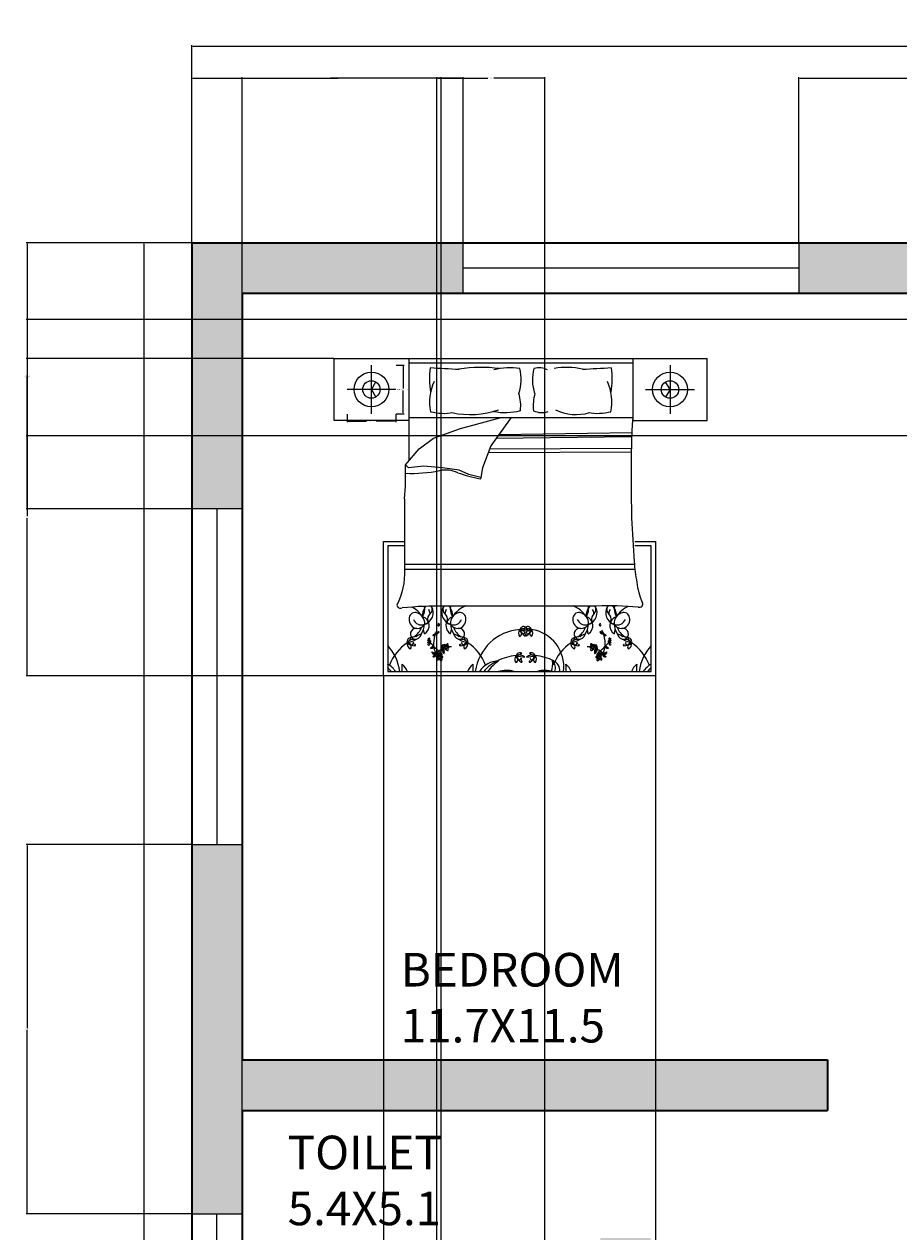
# Model space of a CAD drawing. Units: inches. Extents: x 0 to 423, y -517 to 94.
# Tile 6 of 8: x 0 to 156, y -160 to 55. Entities that reach past the tile are written whole.
import ezdxf

# ---------------------------------------------------------------- set-up
doc = ezdxf.new("R2010")
doc.units = ezdxf.units.IN
doc.header["$MEASUREMENT"] = 0
for name, color, linetype, lineweight in [('A-ANNO-DIMS', 2, 'Continuous', 18), ('A-AREA-IDEN', 7, 'Continuous', 18), ('A-FURN', 8, 'Continuous', 13), ('A-GLAZ', 4, 'Continuous', 18), ('A-WALL', 7, 'Continuous', 35)]:
    doc.layers.add(name, color=color, linetype=linetype, lineweight=lineweight)
doc.layers.add('A-WALL-PATT', color=30, linetype='Continuous', lineweight=13, true_color=0xf26722)
doc.styles.get("Standard").update_dxf_attribs({"font": 'arial.ttf'})
doc.dimstyles.get("Standard").update_dxf_attribs({"dimtxt": 0.18, "dimasz": 0.18, "dimexe": 0.18, "dimexo": 0.0625, "dimgap": 0.09, "dimtad": 0, "dimtih": 1, "dimtoh": 1, "dimdec": 0, "dimzin": 0, "dimdsep": 46, "dimlunit": 3, "dimtxsty": 'Standard', "dimcen": 0.09, "dimadec": 0, "dimazin": 0, "dimtfac": 1, "dimtdec": 0, "dimtofl": 0, "dimtmove": 0, "dimatfit": 3, "dimfxl": 1, "dimtolj": 1, "dimtzin": 0, "dimarcsym": 0})

# ---------------------------------------------------------------- blocks, each defined once
blk = doc.blocks.new('*D1')
at = {"layer": 'A-ANNO-DIMS', "color": 0, "lineweight": -2, "transparency": 16777216}
for p, q in [((29.72, 16.3), (29.72, 51.54)), ((29.9, 51.36), (200.83, 51.36)), ((392.54, 51.36), (221.62, 51.36)), ((392.72, 16.3), (392.72, 51.54))]:
    blk.add_line(p, q, dxfattribs=at)
at = {"layer": 'A-ANNO-DIMS', "color": 0, "transparency": 16777216}
for points in [[(29.9, 51.39), (29.9, 51.33), (29.72, 51.36)], [(392.54, 51.39), (392.54, 51.33), (392.72, 51.36)]]:
    blk.add_solid(points, dxfattribs=at)
at = {"layer": 'Defpoints', "color": 0, "transparency": 16777216}
for p in [(392.72, 51.36), (29.72, 16.23), (392.72, 16.23)]:
    blk.add_point(p, dxfattribs=at)
at = {"layer": 'A-ANNO-DIMS', "color": 0, "transparency": 16777216, "insert": (211.22, 51.36), "char_height": 6, "attachment_point": 5}
blk.add_mtext('\\A1;30\'-3"', dxfattribs=at)
blk = doc.blocks.new('*D2')
at = {"layer": 'A-ANNO-DIMS', "color": 0, "lineweight": -2, "transparency": 16777216}
for p, q in [((29.66, 16.23), (21, 16.23)), ((21.18, 16.05), (21.18, -222.61)), ((21.18, -467.59), (21.18, -228.92)), ((29.66, -467.77), (21, -467.77))]:
    blk.add_line(p, q, dxfattribs=at)
at = {"layer": 'A-ANNO-DIMS', "color": 0, "transparency": 16777216}
for points in [[(21.15, 16.05), (21.21, 16.05), (21.18, 16.23)], [(21.15, -467.59), (21.21, -467.59), (21.18, -467.77)]]:
    blk.add_solid(points, dxfattribs=at)
at = {"layer": 'Defpoints', "color": 0, "transparency": 16777216}
for p in [(29.72, 16.23), (21.18, -467.77), (29.72, -467.77)]:
    blk.add_point(p, dxfattribs=at)
at = {"layer": 'A-ANNO-DIMS', "color": 0, "transparency": 16777216, "insert": (21.18, -225.77), "char_height": 6, "attachment_point": 5}
blk.add_mtext('\\A1;40\'-4"', dxfattribs=at)
blk = doc.blocks.new('WIN-GLAZ-60IN')
for p, q in [((0, 60), (0, 0)), ((4.5, 60), (4.5, 0)), ((9, 0), (9, 60))]:
    blk.add_line(p, q)
blk = doc.blocks.new('WIN-GLAZ-24IN')
for p, q in [((0, 0), (0, 24)), ((4.5, 0), (4.5, 24)), ((9, 24), (9, 0))]:
    blk.add_line(p, q)
blk = doc.blocks.new('BEDSIDE-LAMP-SMALL')
for p, q in [((4.36, 0), (4.36, 8.72)), ((8.72, 4.36), (0, 4.36))]:
    blk.add_line(p, q)
for points in [[(4.36, 4.36), (5.14, 5.71)], [(4.36, 4.36), (5.14, 3.01)]]:
    blk.add_lwpolyline(points)
for radius in [3.11, 1.56]:
    blk.add_circle((4.36, 4.36), radius)
blk = doc.blocks.new('*D24')
at = {"layer": 'A-ANNO-DIMS', "color": 0, "lineweight": -2, "transparency": 16777216}
for p, q in [((66.26, -5.62), (67.69, -5.62)), ((67.51, -5.8), (67.51, -9.79)), ((67.51, -14.15), (67.51, -10.16)), ((66.26, -14.33), (67.69, -14.33))]:
    blk.add_line(p, q, dxfattribs=at)
at = {"layer": 'A-ANNO-DIMS', "color": 0, "transparency": 16777216}
for points in [[(67.48, -5.8), (67.54, -5.8), (67.51, -5.62)], [(67.48, -14.15), (67.54, -14.15), (67.51, -14.33)]]:
    blk.add_solid(points, dxfattribs=at)
at = {"layer": 'Defpoints', "color": 0, "transparency": 16777216}
for p in [(66.2, -5.62), (67.51, -5.62), (66.2, -14.33)]:
    blk.add_point(p, dxfattribs=at)
at = {"layer": 'A-ANNO-DIMS', "color": 0, "transparency": 16777216, "insert": (67.51, -9.98), "char_height": 0.18, "attachment_point": 5}
blk.add_mtext('\\A1;LAMP 0\'-8 1/2" TYP.', dxfattribs=at)
blk = doc.blocks.new('*D25')
at = {"layer": 'A-ANNO-DIMS', "color": 0, "lineweight": -2, "transparency": 16777216}
for p, q in [((57.49, -14.4), (57.49, -15.82)), ((66.2, -14.4), (66.2, -15.82)), ((57.67, -15.64), (60.99, -15.64)), ((66.02, -15.64), (62.69, -15.64))]:
    blk.add_line(p, q, dxfattribs=at)
at = {"layer": 'A-ANNO-DIMS', "color": 0, "transparency": 16777216}
for points in [[(57.67, -15.61), (57.67, -15.67), (57.49, -15.64)], [(66.02, -15.61), (66.02, -15.67), (66.2, -15.64)]]:
    blk.add_solid(points, dxfattribs=at)
at = {"layer": 'Defpoints', "color": 0, "transparency": 16777216}
for p in [(57.49, -14.33), (66.2, -14.33), (66.2, -15.64)]:
    blk.add_point(p, dxfattribs=at)
at = {"layer": 'A-ANNO-DIMS', "color": 0, "transparency": 16777216, "insert": (61.84, -15.64), "char_height": 0.18, "attachment_point": 5}
blk.add_mtext('\\A1;0\'-8 1/2" TYP.', dxfattribs=at)
blk = doc.blocks.new('*D33')
at = {"layer": 'A-ANNO-DIMS', "color": 0, "lineweight": -2, "transparency": 16777216}
for p, q in [((38.72, -374.65), (38.72, 45.81)), ((38.9, 45.63), (55.89, 45.63)), ((74.1, 45.63), (57.11, 45.63)), ((74.28, -374.65), (74.28, 45.81))]:
    blk.add_line(p, q, dxfattribs=at)
at = {"layer": 'A-ANNO-DIMS', "color": 0, "transparency": 16777216}
for points in [[(38.9, 45.66), (38.9, 45.6), (38.72, 45.63)], [(74.1, 45.66), (74.1, 45.6), (74.28, 45.63)]]:
    blk.add_solid(points, dxfattribs=at)
at = {"layer": 'Defpoints', "color": 0, "transparency": 16777216}
for p in [(74.28, 45.63), (38.72, -374.71), (74.28, -374.71)]:
    blk.add_point(p, dxfattribs=at)
at = {"layer": 'A-ANNO-DIMS', "color": 0, "transparency": 16777216, "insert": (56.5, 45.63), "char_height": 0.18, "attachment_point": 5}
blk.add_mtext('\\A1;2\'-11 1/2"', dxfattribs=at)
blk = doc.blocks.new('*D38')
at = {"layer": 'A-ANNO-DIMS', "color": 0, "lineweight": -2, "transparency": 16777216}
for p, q in [((29.72, 16.3), (29.72, 45.81)), ((29.9, 45.63), (53.43, 45.63)), ((78.04, 45.63), (54.52, 45.63)), ((78.22, 16.3), (78.22, 45.81))]:
    blk.add_line(p, q, dxfattribs=at)
at = {"layer": 'A-ANNO-DIMS', "color": 0, "transparency": 16777216}
for points in [[(29.9, 45.66), (29.9, 45.6), (29.72, 45.63)], [(78.04, 45.66), (78.04, 45.6), (78.22, 45.63)]]:
    blk.add_solid(points, dxfattribs=at)
at = {"layer": 'Defpoints', "color": 0, "transparency": 16777216}
for p in [(78.22, 45.63), (29.72, 16.23), (78.22, 16.23)]:
    blk.add_point(p, dxfattribs=at)
at = {"layer": 'A-ANNO-DIMS', "color": 0, "transparency": 16777216, "insert": (53.97, 45.63), "char_height": 0.18, "attachment_point": 5}
blk.add_mtext('\\A1;4\'-0 1/2"', dxfattribs=at)
blk = doc.blocks.new('*D39')
at = {"layer": 'A-ANNO-DIMS', "color": 0, "lineweight": -2, "transparency": 16777216}
for p, q in [((138.22, 16.3), (138.22, 45.81)), ((138.4, 45.63), (169.33, 45.63)), ((201.34, 45.63), (170.41, 45.63)), ((201.52, 16.3), (201.52, 45.81))]:
    blk.add_line(p, q, dxfattribs=at)
at = {"layer": 'A-ANNO-DIMS', "color": 0, "transparency": 16777216}
for points in [[(138.4, 45.66), (138.4, 45.6), (138.22, 45.63)], [(201.34, 45.66), (201.34, 45.6), (201.52, 45.63)]]:
    blk.add_solid(points, dxfattribs=at)
at = {"layer": 'Defpoints', "color": 0, "transparency": 16777216}
for p in [(201.52, 45.63), (138.22, 16.23), (201.52, 16.23)]:
    blk.add_point(p, dxfattribs=at)
at = {"layer": 'A-ANNO-DIMS', "color": 0, "transparency": 16777216, "insert": (169.87, 45.63), "char_height": 0.18, "attachment_point": 5}
blk.add_mtext('\\A1;5\'-3 1/2"', dxfattribs=at)
blk = doc.blocks.new('*D41')
at = {"layer": 'A-ANNO-DIMS', "color": 0, "lineweight": -2, "transparency": 16777216}
for p, q in [((29.66, 16.23), (0.14, 16.23)), ((0.32, 16.05), (0.32, -7.33)), ((0.32, -31.09), (0.32, -7.7)), ((29.66, -31.27), (0.14, -31.27))]:
    blk.add_line(p, q, dxfattribs=at)
at = {"layer": 'A-ANNO-DIMS', "color": 0, "transparency": 16777216}
for points in [[(0.29, 16.05), (0.35, 16.05), (0.32, 16.23)], [(0.29, -31.09), (0.35, -31.09), (0.32, -31.27)]]:
    blk.add_solid(points, dxfattribs=at)
at = {"layer": 'Defpoints', "color": 0, "transparency": 16777216}
for p in [(0.32, 16.23), (29.72, 16.23), (29.72, -31.27)]:
    blk.add_point(p, dxfattribs=at)
at = {"layer": 'A-ANNO-DIMS', "color": 0, "transparency": 16777216, "insert": (0.32, -7.52), "char_height": 0.18, "attachment_point": 5}
blk.add_mtext('\\A1;3\'-11 1/2"', dxfattribs=at)
blk = doc.blocks.new('*D45')
at = {"layer": 'A-ANNO-DIMS', "color": 0, "lineweight": -2, "transparency": 16777216}
for p, q in [((29.66, -91.27), (0.14, -91.27)), ((0.32, -91.45), (0.32, -124.08)), ((0.32, -157.09), (0.32, -124.45)), ((29.66, -157.27), (0.14, -157.27))]:
    blk.add_line(p, q, dxfattribs=at)
at = {"layer": 'A-ANNO-DIMS', "color": 0, "transparency": 16777216}
for points in [[(0.29, -91.45), (0.35, -91.45), (0.32, -91.27)], [(0.29, -157.09), (0.35, -157.09), (0.32, -157.27)]]:
    blk.add_solid(points, dxfattribs=at)
at = {"layer": 'Defpoints', "color": 0, "transparency": 16777216}
for p in [(0.32, -91.27), (29.72, -91.27), (29.72, -157.27)]:
    blk.add_point(p, dxfattribs=at)
at = {"layer": 'A-ANNO-DIMS', "color": 0, "transparency": 16777216, "insert": (0.32, -124.27), "char_height": 0.18, "attachment_point": 5}
blk.add_mtext('\\A1;5\'-6"', dxfattribs=at)
blk = doc.blocks.new('*D49')
at = {"layer": 'A-ANNO-DIMS', "color": 0, "lineweight": -2, "transparency": 16777216}
for p, q in [((63.98, -61.2), (63.98, -517.35)), ((112.6, -61.2), (112.6, -517.35)), ((64.16, -517.17), (87.75, -517.17)), ((112.42, -517.17), (88.83, -517.17))]:
    blk.add_line(p, q, dxfattribs=at)
at = {"layer": 'A-ANNO-DIMS', "color": 0, "transparency": 16777216}
for points in [[(64.16, -517.14), (64.16, -517.2), (63.98, -517.17)], [(112.42, -517.14), (112.42, -517.2), (112.6, -517.17)]]:
    blk.add_solid(points, dxfattribs=at)
at = {"layer": 'Defpoints', "color": 0, "transparency": 16777216}
for p in [(63.98, -61.14), (112.6, -61.14), (112.6, -517.17)]:
    blk.add_point(p, dxfattribs=at)
at = {"layer": 'A-ANNO-DIMS', "color": 0, "transparency": 16777216, "insert": (88.29, -517.17), "char_height": 0.18, "attachment_point": 5}
blk.add_mtext('\\A1;4\'-0 1/2"', dxfattribs=at)
blk = doc.blocks.new('*D52')
at = {"layer": 'A-ANNO-DIMS', "color": 0, "lineweight": -2, "transparency": 16777216}
for p, q in [((73.55, -270.94), (73.55, 45.81)), ((73.73, 45.63), (82.66, 45.63)), ((92.66, 45.63), (83.72, 45.63)), ((92.84, -254.62), (92.84, 45.81))]:
    blk.add_line(p, q, dxfattribs=at)
at = {"layer": 'A-ANNO-DIMS', "color": 0, "transparency": 16777216}
for points in [[(73.73, 45.66), (73.73, 45.6), (73.55, 45.63)], [(92.66, 45.66), (92.66, 45.6), (92.84, 45.63)]]:
    blk.add_solid(points, dxfattribs=at)
at = {"layer": 'Defpoints', "color": 0, "transparency": 16777216}
for p in [(92.84, 45.63), (92.84, -254.68), (73.55, -271)]:
    blk.add_point(p, dxfattribs=at)
at = {"layer": 'A-ANNO-DIMS', "color": 0, "transparency": 16777216, "insert": (83.19, 45.63), "char_height": 0.18, "attachment_point": 5}
blk.add_mtext('\\A1;1\'-7 1/2"', dxfattribs=at)
blk = doc.blocks.new('*D59')
at = {"layer": 'A-ANNO-DIMS', "color": 0, "lineweight": -2, "transparency": 16777216}
for p, q in [((55.11, -4.42), (0.14, -4.42)), ((0.32, -4.6), (0.32, -32.6)), ((0.32, -60.96), (0.32, -32.96)), ((63.91, -61.14), (0.14, -61.14))]:
    blk.add_line(p, q, dxfattribs=at)
at = {"layer": 'A-ANNO-DIMS', "color": 0, "transparency": 16777216}
for points in [[(0.29, -4.6), (0.35, -4.6), (0.32, -4.42)], [(0.29, -60.96), (0.35, -60.96), (0.32, -61.14)]]:
    blk.add_solid(points, dxfattribs=at)
at = {"layer": 'Defpoints', "color": 0, "transparency": 16777216}
for p in [(55.17, -4.42), (0.32, -61.14), (63.98, -61.14)]:
    blk.add_point(p, dxfattribs=at)
at = {"layer": 'A-ANNO-DIMS', "color": 0, "transparency": 16777216, "insert": (0.32, -32.78), "char_height": 0.18, "attachment_point": 5}
blk.add_mtext('\\A1;4\'-8 1/2"', dxfattribs=at)
blk = doc.blocks.new('*D63')
at = {"layer": 'A-ANNO-DIMS', "color": 0, "lineweight": -2, "transparency": 16777216}
for p, q in [((256.66, 2.55), (0.14, 2.55)), ((0.32, 2.37), (0.32, -7.66)), ((0.32, -18.06), (0.32, -8.03)), ((256.66, -18.24), (0.14, -18.24))]:
    blk.add_line(p, q, dxfattribs=at)
at = {"layer": 'A-ANNO-DIMS', "color": 0, "transparency": 16777216}
for points in [[(0.29, 2.37), (0.35, 2.37), (0.32, 2.55)], [(0.29, -18.06), (0.35, -18.06), (0.32, -18.24)]]:
    blk.add_solid(points, dxfattribs=at)
at = {"layer": 'Defpoints', "color": 0, "transparency": 16777216}
for p in [(256.72, 2.55), (0.32, -18.24), (256.72, -18.24)]:
    blk.add_point(p, dxfattribs=at)
at = {"layer": 'A-ANNO-DIMS', "color": 0, "transparency": 16777216, "insert": (0.32, -7.84), "char_height": 0.18, "attachment_point": 5}
blk.add_mtext('\\A1;1\'-9"', dxfattribs=at)

msp = doc.modelspace()

# ---------------------------------------------------------------- hatches: boundary and pattern name
at = {"layer": 'A-WALL-PATT'}
h = msp.add_hatch(color=256, dxfattribs=at)
h.dxf.hatch_style = 1
h.paths.add_polyline_path([(201.52, 16.23), (138.22, 16.23), (138.22, 7.23), (177.72, 7.23), (177.72, -138.77), (186.72, -138.77), (186.72, -92.77), (251.72, -92.77), (251.72, -22.53), (242.72, -22.53), (242.72, -83.77), (186.72, -83.77), (186.72, 7.23), (201.52, 7.23)])
h.paths.add_polyline_path([(78.22, 16.23), (29.72, 16.23), (29.72, -31.27), (38.72, -31.27), (38.72, 7.23), (78.22, 7.23)])
h.paths.add_polyline_path([(275.31, 16.23), (225.52, 16.23), (225.52, 7.23), (275.31, 7.23)])
h.paths.add_polyline_path([(392.72, 16.23), (335.31, 16.23), (335.31, 7.23), (383.72, 7.23), (383.72, -31.27), (392.72, -31.27)])
h.paths.add_polyline_path([(143.33, -129.77), (38.72, -129.77), (38.72, -91.27), (29.72, -91.27), (29.72, -157.27), (38.72, -157.27), (38.72, -138.77), (143.33, -138.77)])
h.paths.add_polyline_path([(186.72, -199.77), (38.72, -199.77), (38.72, -181.27), (29.72, -181.27), (29.72, -239.27), (38.72, -239.27), (38.72, -208.77), (177.72, -208.77), (177.72, -237.07), (186.72, -237.07)])
h.paths.add_polyline_path([(111.72, -161.55), (102.72, -161.55), (102.72, -199.77), (111.72, -199.77)])
h.paths.add_polyline_path([(392.72, -91.27), (383.72, -91.27), (383.72, -129.77), (242.72, -129.77), (242.72, -138.77), (383.72, -138.77), (383.72, -169.77), (392.72, -169.77)])
h.paths.add_polyline_path([(392.72, -229.77), (383.72, -229.77), (383.72, -262.77), (251.72, -262.77), (251.72, -177.14), (242.72, -177.14), (242.72, -271.77), (383.72, -271.77), (383.72, -300.77), (392.72, -300.77)])
h.paths.add_polyline_path([(392.72, -360.77), (383.72, -360.77), (383.72, -389.77), (378.42, -389.77), (378.42, -398.77), (383.72, -398.77), (383.72, -458.77), (382.72, -458.77), (382.72, -467.77), (392.72, -467.77)])
h.paths.add_polyline_path([(364.92, -389.77), (348.72, -389.77), (348.72, -467.77), (358.72, -467.77), (358.72, -458.77), (357.72, -458.77), (357.72, -398.77), (364.92, -398.77)])
h.paths.add_polyline_path([(320.72, -389.77), (283.72, -389.77), (283.72, -398.77), (320.72, -398.77)])
h.paths.add_polyline_path([(223.72, -389.77), (186.72, -389.77), (186.72, -270.38), (177.72, -270.38), (177.72, -458.77), (138.22, -458.77), (138.22, -467.77), (186.72, -467.77), (186.72, -398.77), (223.72, -398.77)])
h.paths.add_polyline_path([(143.29, -329.77), (38.72, -329.77), (38.72, -299.27), (29.72, -299.27), (29.72, -338.77), (143.29, -338.77)])
h.paths.add_polyline_path([(38.72, -374.71), (29.72, -374.71), (29.72, -398.74), (38.72, -398.74)])
h.paths.add_polyline_path([(78.22, -458.77), (38.72, -458.77), (38.72, -434.74), (29.72, -434.74), (29.72, -467.77), (78.22, -467.77)])
h.paths.add_polyline_path([(279.99, -158.17), (326.6, -158.17), (326.6, -135.78), (279.99, -135.78)], flags=25)
h.paths.add_polyline_path([(355.56, -439.13), (387, -439.13), (387, -416.66), (355.56, -416.66)], flags=9)

# ---------------------------------------------------------------- linework, layer by layer
at = {"layer": 'A-FURN'}
for p, q in [((55.17, -4.42), (121.87, -4.42)), ((68.51, -4.42), (68.51, -22.72)), ((108.53, -5.27), (68.51, -5.27)), ((68.51, -14.96), (108.53, -14.96)), ((77.78, -16.94), (85.05, -14.96)), ((86.84, -14.96), (83.18, -20.05)), ((72.91, -18.7), (77.78, -16.94)), ((70.35, -20.59), (72.91, -18.7)), ((108.33, -18.41), (84.11, -18.76)), ((108.35, -17.73), (84.61, -18.06)), ((67.92, -23.42), (70.35, -20.59)), ((83.18, -20.05), (81.7, -23.96)), ((108.3, -21.2), (82.7, -21.3)), ((108.29, -20.51), (82.97, -20.61)), ((68.46, -23.96), (67.92, -23.42)), ((71.16, -23.69), (68.46, -23.96)), ((74.54, -23.96), (71.16, -23.69)), ((77.51, -24.37), (74.54, -23.96)), ((79.26, -25.18), (77.51, -24.37)), ((81.42, -25.72), (79.26, -25.18)), ((81.7, -23.96), (81.42, -25.72)), ((63.98, -37.11), (67.75, -37.11)), ((63.98, -61.14), (63.98, -37.11)), ((67.75, -37.89), (64.75, -37.89)), ((64.75, -37.89), (64.75, -60.37)), ((111.83, -37.89), (108.89, -37.89)), ((108.9, -37.11), (112.6, -37.11)), ((111.83, -60.37), (111.83, -37.89)), ((112.6, -37.11), (112.6, -61.14)), ((108.83, -41.27), (67.74, -41.27)), ((108.9, -42.11), (67.74, -42.11)), ((102.06, -48.66), (74.98, -48.66)), ((71.32, -53.61), (71.17, -52.85)), ((75.98, -53.61), (76.13, -52.85)), ((100.6, -53.61), (100.45, -52.85)), ((105.26, -53.61), (105.4, -52.85)), ((64.75, -60.37), (111.83, -60.37)), ((112.6, -61.14), (63.98, -61.14))]:
    msp.add_line(p, q, dxfattribs=at)
for points in [[(68.51, -15.53), (55.17, -15.53), (55.17, -4.42)], [(108.53, -4.42), (108.53, -15.53), (121.87, -15.53), (121.87, -4.42)]]:
    msp.add_lwpolyline(points, dxfattribs=at)
for points in [[(72.34, -6.08, 0.074897), (72.42, -10.44, -0.472817)], [(88.21, -10.68, 0.14099), (88.34, -6.24, 0.235245)], [(91.06, -10.68, -0.14099), (90.92, -6.24, -0.235245)], [(104.7, -6.08, -0.074897), (104.62, -10.44, 0.472817)], [(67.78, -29.53, 0.001242), (67.74, -42.18, -0.127202), (66.41, -48.49)], [(108.82, -40.75, 0.056112), (109.3, -44.42, 0.095341), (110.24, -47.95)]]:
    msp.add_lwpolyline(points, format="xyb", dxfattribs=at)
for centre in [(75.18, -56.02), (101.4, -56.02), (74.06, -57.81), (102.51, -57.81)]:
    msp.add_circle(centre, 0.17, dxfattribs=at)
for centre, radius, start, end in [((109.11, 628.67), 635.81, 266.68521, 267.14978), ((81.48, -30.22), 24.19, 82.2196, 99.497), ((86.59, -17.99), 11.88, 81.5249, 103.96), ((91.84, -9.41), 3.3, 63.3437, 106.1026), ((96.78, -17.75), 11.73, 76.3427, 101.1841), ((67.94, 628.67), 635.81, 272.85022, 273.31479), ((80.84, -12.19), 8.6, 155.1316, 191.7583), ((96.2, -12.19), 8.6, 348.2417, 24.8684), ((80.35, -12.91), 8.17, 354.0129, 15.8293), ((98.92, -12.91), 8.17, 164.1707, 185.9871), ((74.72, -5.3), 8.94, 255.1039, 281.0369), ((79.43, 1.05), 15.5, 258.0397, 289.2615), ((85.7, -2.33), 11.76, 259.8617, 283.6238), ((92.29, -10.56), 3.54, 245.0183, 288.5407), ((98.46, -5.96), 8.49, 243.8761, 286.1746), ((102.32, -5.3), 8.94, 258.9631, 284.8961), ((228.1, -23.11), 119.85, 176.1, 180.9282), ((6.76, -25.08), 61.18, 355.8294, 1.553), ((69.06, 0.2), 25.17, 267.4519, 281.3392), ((75.07, -29.81), 5.43, 66.2616, 101.3392), ((86.06, -0.51), 25.87, 250.1194, 259.3383), ((81.27, -25.77), 0.161, 268.8623, 19.7536), ((264.58, -27.47), 156.33, 179.1145, 184.8735), ((67.02, -48.45), 0.615, 183.98, 297.3412), ((74.19, -118.09), 69.43, 89.3433, 95.6887), ((66.76, -53.35), 5.05, 33.6671, 63.2997), ((73.53, -50.35), 2.57, 145.785, 184.7304), ((68.61, -49.15), 2.76, 328.8218, 9.1554), ((72.03, -49.4), 0.803, 120.0293, 142.325), ((70.75, -49.87), 2.13, 289.2822, 29.1751), ((70.43, -50.25), 1.92, 7.436, 29.9149), ((71.7, -49.24), 0.998, 311.5653, 23.8354), ((72.03, -49.4), 0.803, 44.4517, 63.558), ((76.55, -49.87), 2.13, 150.8249, 250.7178), ((75.61, -49.24), 0.998, 156.1646, 228.4347), ((75.27, -49.4), 0.803, 113.229, 135.5483), ((76.87, -50.25), 1.92, 150.0851, 172.564), ((75.27, -49.4), 0.803, 37.675, 66.7144), ((73.78, -50.35), 2.57, 355.2696, 34.215), ((78.69, -49.15), 2.76, 169.7133, 211.1782), ((80.55, -53.35), 5.05, 111.4941, 146.3329), ((96.03, -53.35), 5.05, 33.6671, 68.5059), ((102.8, -50.35), 2.57, 145.785, 184.7304), ((97.89, -49.15), 2.76, 328.8218, 10.2867), ((101.31, -49.4), 0.803, 113.2856, 142.325), ((100.03, -49.87), 2.13, 289.2822, 29.1751), ((99.7, -50.25), 1.92, 7.436, 29.9149), ((101.31, -49.4), 0.803, 44.4517, 66.7144), ((100.97, -49.24), 0.998, 311.5653, 23.8354), ((104.11, -113.53), 64.9, 85.2402, 91.8035), ((105.83, -49.87), 2.13, 150.8249, 250.7178), ((104.88, -49.24), 0.998, 156.1646, 228.4347), ((104.54, -49.4), 0.803, 106.6343, 135.5483), ((106.15, -50.25), 1.92, 150.0851, 172.564), ((104.54, -49.4), 0.803, 37.675, 72.5814), ((103.05, -50.35), 2.57, 355.2696, 34.215), ((107.97, -49.15), 2.76, 169.249, 211.1782), ((109.82, -53.35), 5.05, 113.6453, 146.3329), ((109.73, -48.29), 0.608, 246.5219, 33.8264), ((70.16, -51.09), 1.59, 174.9449, 262.8857), ((69.7, -50.93), 1.13, 84.4856, 181.0538), ((70.79, -50.49), 1.55, 201.5819, 291.4221), ((69.36, -51.76), 2.01, 355.2933, 76.921), ((70.5, -52.17), 1.66, 299.9085, 73.1337), ((73.53, -50.35), 2.57, 212.7011, 216.3445), ((71.55, -51.47), 0.414, 257.3041, 15.1471), ((73.26, -51.01), 1.37, 131.5653, 195.1471), ((74.04, -51.01), 1.37, 344.8529, 48.4347), ((76.81, -52.17), 1.66, 106.8663, 240.0915), ((75.76, -51.47), 0.414, 164.8529, 282.6959), ((73.78, -50.35), 2.57, 323.6555, 327.2989), ((77.95, -51.76), 2.01, 103.079, 184.7067), ((76.52, -50.49), 1.55, 248.5779, 338.4181), ((77.14, -51.09), 1.59, 277.1143, 5.0551), ((77.6, -50.93), 1.13, 358.9462, 95.5144), ((99.44, -51.09), 1.59, 174.9449, 262.8857), ((98.97, -50.93), 1.13, 84.4856, 181.0538), ((100.06, -50.49), 1.55, 201.5819, 291.4221), ((98.63, -51.76), 2.01, 355.2933, 76.921), ((99.77, -52.17), 1.66, 299.9085, 73.1337), ((102.8, -50.35), 2.57, 212.7011, 216.3445), ((100.82, -51.47), 0.414, 257.3041, 15.1471), ((102.54, -51.01), 1.37, 131.5653, 195.1471), ((103.31, -51.01), 1.37, 344.8529, 48.4347), ((106.08, -52.17), 1.66, 106.8663, 240.0915), ((105.03, -51.47), 0.414, 164.8529, 282.6959), ((103.05, -50.35), 2.57, 323.6555, 327.2989), ((107.22, -51.76), 2.01, 103.079, 184.7067), ((105.79, -50.49), 1.55, 248.5779, 338.4181), ((106.42, -51.09), 1.59, 277.1143, 5.0551), ((106.88, -50.93), 1.13, 358.9462, 95.5144), ((69.8, -53.66), 1, 80.264, 250.8688), ((67.81, -51.46), 3.15, 301.2614, 341.7045), ((69.56, -53.36), 1.25, 265.969, 344.3045), ((70.9, -55.02), 1.33, 96.1662, 141.5825), ((69.89, -50.74), 1.94, 272.3591, 324.0401), ((67.78, -51.71), 3.58, 326.2883, 356.5076), ((73.11, -54.09), 0.35, 101.3256, 154.4621), ((72.6, -52.9), 1.05, 280.2588, 300.656), ((72.85, -52.06), 1.88, 268.3264, 277.1302), ((78.47, -55.46), 5.52, 163.5842, 183.8277), ((72.38, -52.9), 1.07, 308.2101, 316.3071), ((73.03, -53.6), 0.32, 278.3432, 4.2869), ((72.86, -53.32), 0.559, 300.656, 332.6341), ((73.28, -53.69), 0.136, 55.7657, 157.4417), ((78.47, -55.46), 5.52, 153.0032, 159.8941), ((73.49, -53.57), 0.136, 84.3784, 186.0543), ((73.36, -53.02), 0.559, 269.1859, 301.164), ((73.52, -53.31), 0.32, 237.5332, 323.4768), ((73.21, -52.4), 1.07, 285.5129, 293.6099), ((73.91, -53.6), 0.35, 87.3579, 140.4944), ((73.1, -52.6), 1.05, 301.164, 321.5612), ((73.84, -52.1), 0.129, 102.7051, 280.4384), ((72.25, -52.41), 1.88, 324.6898, 333.4936), ((73.83, -52.02), 0.209, 280.4384, 100.4136), ((77.42, -50.74), 1.94, 215.9599, 267.6409), ((79.52, -51.71), 3.58, 183.4924, 213.7117), ((79.49, -51.46), 3.15, 198.2955, 238.7386), ((76.4, -55.02), 1.33, 38.4175, 83.8338), ((77.75, -53.36), 1.25, 195.6955, 274.031), ((77.51, -53.66), 1, 289.1312, 99.736), ((89.04, -61.54), 8.71, 94.4623, 172.255), ((89.08, -53.51), 0.966, 137.7873, 219.1145), ((87.98, -53.48), 0.727, 298.5391, 58.3627), ((89.06, -53.06), 0.722, 63.0274, 163.8037), ((88.33, -51.37), 1.49, 271.4585, 315.3727), ((88.93, -54.11), 1.38, 45.5411, 114.3101), ((90.19, -47.04), 6.09, 252.593, 267.2582), ((89.08, -52.89), 0.713, 177.7585, 283.852), ((90.45, -52.14), 2.2, 198.9159, 238.011), ((89.87, -54.11), 1.38, 65.6899, 134.4589), ((88.62, -47.04), 6.09, 272.7418, 287.407), ((89.22, -53.49), 0.0942, 283.852, 219.9245), ((89.34, -53.92), 0.108, 238.011, 71.5592), ((89.35, -53.87), 0.0525, 71.5592, 188.0167), ((89.47, -53.92), 0.108, 108.4408, 301.989), ((89.75, -53.06), 0.722, 16.1963, 116.9726), ((90.48, -51.37), 1.49, 224.6273, 268.5415), ((89.45, -53.87), 0.0525, 351.9833, 108.4408), ((89.57, -53.45), 0.0568, 320.1909, 256.0209), ((88.36, -52.14), 2.2, 301.989, 341.0841), ((89.73, -52.89), 0.713, 256.148, 2.2415), ((90.82, -53.48), 0.727, 121.6373, 241.4609), ((89.72, -53.51), 0.966, 320.8855, 42.2127), ((89.48, -59.53), 6.74, 352.8636, 81.8197), ((99.07, -53.66), 1, 80.264, 250.8688), ((97.09, -51.46), 3.15, 301.2614, 341.7045), ((98.83, -53.36), 1.25, 265.969, 344.3045), ((100.18, -55.02), 1.33, 96.1662, 141.5825), ((99.16, -50.74), 1.94, 272.3591, 324.0401), ((97.06, -51.71), 3.58, 326.2883, 356.5076), ((102.75, -52.02), 0.209, 79.5864, 259.5616), ((103.47, -52.6), 1.05, 218.4388, 238.836), ((102.66, -53.6), 0.35, 39.5056, 92.6421), ((104.33, -52.41), 1.88, 206.5064, 215.3102), ((102.73, -52.1), 0.129, 259.5616, 77.2949), ((103.05, -53.31), 0.32, 216.5232, 302.4668), ((103.36, -52.4), 1.07, 246.3901, 254.4871), ((103.22, -53.02), 0.559, 238.836, 270.8141), ((98.11, -55.46), 5.52, 20.1059, 26.9968), ((103.09, -53.57), 0.136, 353.9457, 95.6216), ((103.3, -53.69), 0.136, 22.5583, 124.2343), ((103.55, -53.6), 0.32, 175.7131, 261.6568), ((103.72, -53.32), 0.559, 207.3659, 239.344), ((98.11, -55.46), 5.52, 356.1723, 16.4158), ((104.2, -52.9), 1.07, 223.6929, 231.7899), ((103.97, -52.9), 1.05, 239.344, 259.7412), ((103.73, -52.06), 1.88, 262.8698, 271.6736), ((103.47, -54.09), 0.35, 25.5379, 78.6744), ((106.69, -50.74), 1.94, 215.9599, 267.6409), ((108.8, -51.71), 3.58, 183.4924, 213.7117), ((108.77, -51.46), 3.15, 198.2955, 238.7386), ((107.02, -53.36), 1.25, 195.6955, 274.031), ((105.68, -55.02), 1.33, 38.4175, 83.8338), ((106.78, -53.66), 1, 289.1312, 99.736), ((58.27, -61.54), 8.71, 7.745, 41.8856), ((73.17, -62.4), 8.71, 124.3865, 158.5908), ((68.95, -55.04), 0.722, 92.9516, 193.728), ((69.19, -55.42), 0.966, 167.7115, 249.0387), ((67.47, -53.94), 1.49, 301.3827, 345.2969), ((69.36, -56.02), 1.38, 75.4653, 144.2343), ((66.93, -49.27), 6.09, 282.5173, 297.1824), ((68.23, -55.94), 0.727, 328.4633, 88.2869), ((69.7, -53.56), 2.2, 228.8402, 267.9352), ((68.88, -54.88), 0.713, 207.6827, 313.7762), ((69.59, -54.74), 0.614, 63.9755, 143.2681), ((69.31, -55.33), 0.0942, 313.7762, 249.7183), ((69.61, -55.6), 0.0525, 101.4834, 217.9409), ((69.62, -55.65), 0.108, 267.9352, 101.4834), ((72.12, -54.75), 0.283, 101.5637, 142.6358), ((71.88, -55.01), 0.17, 273.2768, 86.7232), ((72.11, -55.33), 0.28, 217.7621, 259.0403), ((72.08, -54.85), 0.162, 91.1081, 181.8675), ((72.42, -54.95), 0.516, 203.4276, 227.6104), ((72.25, -55.18), 0.351, 80.3487, 133.6538), ((72.19, -54.89), 0.278, 229.7889, 317.6792), ((71.89, -54.53), 0.408, 288.7263, 352.5032), ((71.88, -55.48), 0.395, 355.053, 68.3618), ((72.19, -55.54), 0.556, 83.0852, 105.7171), ((72.17, -54.55), 0.131, 345.2356, 144.9248), ((72.14, -55.5), 0.13, 232.4737, 355.053), ((68.34, -60.16), 6.33, 43.1541, 52.0459), ((72.29, -54.98), 0.146, 317.6792, 80.3487), ((72.71, -56.33), 0.35, 101.3256, 154.4621), ((72.21, -55.14), 1.05, 280.2588, 300.656), ((71.98, -55.15), 1.07, 308.2101, 316.3071), ((72.64, -55.85), 0.32, 278.3432, 4.2869), ((72.46, -55.57), 0.559, 300.656, 332.6341), ((72.88, -55.94), 0.136, 55.7657, 157.4417), ((75.72, -55.6), 2.77, 184.756, 209.2041), ((79.7, -49.7), 9.11, 222.2412, 232.1744), ((73.88, -55.77), 0.774, 304.5369, 16.3699), ((74.29, -55.94), 0.471, 272.8499, 356.1226), ((73.96, -56.13), 0.456, 321.7607, 7.9252), ((74.95, -55.99), 0.548, 127.3105, 187.9252), ((74.2, -55.93), 0.563, 355.0106, 41.658), ((75.13, -56.54), 0.536, 104.7558, 148.0499), ((74.99, -55.79), 0.232, 126.1046, 271.4281), ((74.96, -55.72), 0.166, 353.7526, 131.7054), ((74.81, -55.92), 0.234, 0.0645, 61.1507), ((74.86, -55.72), 0.267, 311.8413, 355.7877), ((75.41, -55.76), 0.283, 101.5637, 176.365), ((75.37, -55.86), 0.162, 91.1081, 181.8675), ((75.55, -56.19), 0.351, 80.3487, 133.6538), ((75.48, -55.9), 0.278, 229.7889, 317.6792), ((75.18, -55.54), 0.408, 288.7263, 352.5032), ((75.48, -56.55), 0.556, 83.0852, 105.7171), ((75.46, -55.56), 0.131, 345.2356, 144.9248), ((75.58, -55.99), 0.146, 317.6792, 80.3487), ((76, -59.27), 3.32, 87.1071, 94.7585), ((77.72, -54.74), 0.614, 36.7319, 116.0245), ((77.68, -55.65), 0.108, 78.5166, 272.0648), ((77.94, -56.02), 1.38, 35.7657, 104.5347), ((80.38, -49.27), 6.09, 242.8176, 257.4827), ((77.61, -53.56), 2.2, 272.0648, 311.1598), ((77.7, -55.6), 0.0525, 322.0591, 78.5166), ((78.43, -54.88), 0.713, 226.2238, 332.3173), ((78.01, -55.29), 0.0568, 290.2667, 226.2271), ((79.08, -55.94), 0.727, 91.7131, 211.5367), ((78.36, -55.04), 0.722, 346.272, 87.0484), ((79.83, -53.94), 1.49, 194.7031, 238.6173), ((78.11, -55.42), 0.966, 290.9613, 12.2885), ((74.14, -62.4), 8.71, 21.4092, 55.6135), ((102.44, -62.4), 8.71, 124.3865, 158.5908), ((98.22, -55.04), 0.722, 92.9516, 193.728), ((98.46, -55.42), 0.966, 167.7115, 249.0387), ((96.75, -53.94), 1.49, 301.3827, 345.2969), ((98.64, -56.02), 1.38, 75.4653, 144.2343), ((96.2, -49.27), 6.09, 282.5173, 297.1824), ((98.15, -54.88), 0.713, 207.6827, 313.7762), ((98.97, -53.56), 2.2, 228.8402, 267.9352), ((97.5, -55.94), 0.727, 328.4633, 88.2869), ((98.86, -54.74), 0.614, 63.9755, 143.2681), ((98.58, -55.33), 0.0942, 313.7762, 249.7183), ((98.88, -55.6), 0.0525, 101.4834, 217.9409), ((98.89, -55.65), 0.108, 267.9352, 101.4834), ((100.58, -59.27), 3.32, 85.2415, 92.8929), ((101, -55.99), 0.146, 99.6513, 222.3208), ((101.1, -55.9), 0.278, 222.3208, 310.2111), ((101.03, -56.19), 0.351, 46.3462, 99.6513), ((101.12, -55.56), 0.131, 35.0752, 194.7644), ((101.4, -55.54), 0.408, 187.4968, 251.2737), ((101.1, -56.55), 0.556, 74.2829, 96.9148), ((101.21, -55.86), 0.162, 358.1325, 88.8919), ((101.17, -55.76), 0.283, 3.635, 78.4363), ((101.62, -55.72), 0.166, 48.2946, 186.2474), ((101.72, -55.72), 0.267, 184.2123, 228.1587), ((101.77, -55.92), 0.234, 118.8493, 179.9355), ((101.59, -55.79), 0.232, 268.5719, 53.8954), ((101.45, -56.54), 0.536, 31.9501, 75.2442), ((102.38, -55.93), 0.563, 138.342, 184.9894), ((102.29, -55.94), 0.471, 183.8774, 267.1501), ((102.7, -55.77), 0.774, 163.6301, 235.4631), ((101.63, -55.99), 0.548, 352.0748, 52.6895), ((102.62, -56.13), 0.456, 172.0748, 218.2393), ((96.88, -49.7), 9.11, 307.8256, 317.7588), ((100.86, -55.6), 2.77, 330.7959, 355.244), ((108.24, -60.16), 6.33, 127.9541, 136.8459), ((103.7, -55.94), 0.136, 22.5583, 124.2343), ((103.94, -55.85), 0.32, 175.7131, 261.6568), ((104.12, -55.57), 0.559, 207.3659, 239.344), ((104.6, -55.15), 1.07, 223.6929, 231.7899), ((104.37, -55.14), 1.05, 239.344, 259.7412), ((103.87, -56.33), 0.35, 25.5379, 78.6744), ((104.29, -54.98), 0.146, 99.6513, 222.3208), ((104.39, -54.89), 0.278, 222.3208, 310.2111), ((104.33, -55.18), 0.351, 46.3462, 99.6513), ((104.41, -54.55), 0.131, 35.0752, 194.7644), ((104.69, -54.53), 0.408, 187.4968, 251.2737), ((104.7, -55.48), 0.395, 111.6382, 184.947), ((104.44, -55.5), 0.13, 184.947, 307.5263), ((104.39, -55.54), 0.556, 74.2829, 96.9148), ((104.5, -54.85), 0.162, 358.1325, 88.8919), ((104.16, -54.95), 0.516, 312.3896, 336.5724), ((104.46, -54.75), 0.283, 37.3642, 78.4363), ((104.46, -55.33), 0.28, 280.9597, 322.2379), ((104.7, -55.01), 0.17, 93.2768, 266.7232), ((106.99, -54.74), 0.614, 36.7319, 116.0245), ((106.96, -55.65), 0.108, 78.5166, 272.0648), ((107.21, -56.02), 1.38, 35.7657, 104.5347), ((109.65, -49.27), 6.09, 242.8176, 257.4827), ((106.88, -53.56), 2.2, 272.0648, 311.1598), ((106.97, -55.6), 0.0525, 322.0591, 78.5166), ((107.7, -54.88), 0.713, 226.2238, 332.3173), ((107.28, -55.29), 0.0568, 290.2667, 226.2271), ((108.35, -55.94), 0.727, 91.7131, 211.5367), ((109.11, -53.94), 1.49, 194.7031, 238.6173), ((107.63, -55.04), 0.722, 346.272, 87.0484), ((107.39, -55.42), 0.966, 290.9613, 12.2885), ((103.41, -62.4), 8.71, 21.4092, 55.6135), ((118.31, -61.54), 8.71, 138.1144, 172.255), ((72.45, -54.3), 1.88, 268.3264, 277.1302), ((72.83, -56.94), 0.19, 146.8636, 236.9021), ((75.5, -52.77), 4.96, 235.1882, 238.8844), ((73.15, -56.67), 0.513, 199.4799, 267.6828), ((73.1, -56.86), 0.442, 212.8155, 277.3992), ((72.84, -57.16), 0.513, 266.9701, 338.2913), ((70.13, -53.5), 4.96, 302.6784, 306.3746), ((72.97, -57.57), 0.19, 214.3538, 304.3923), ((73.04, -56.85), 0.196, 238.8844, 314.2646), ((73, -57.29), 0.442, 280.3057, 17.1958), ((72.96, -57.33), 0.196, 306.3746, 21.7548), ((73.28, -57.21), 0.148, 19.3605, 201.7548), ((73.28, -57.09), 0.148, 311.8703, 134.2646), ((76.07, -58.44), 2.96, 153.7819, 158.2913), ((73.71, -56.42), 0.774, 247.2305, 319.0635), ((73.46, -56.68), 0.456, 264.4544, 310.6188), ((75.72, -55.6), 2.77, 214.0033, 222.4917), ((73.79, -56.86), 0.471, 218.3208, 298.8162), ((76, -59.27), 3.32, 120.544, 139.818), ((73.71, -58.13), 0.168, 148.0499, 225.6268), ((74.02, -58.33), 0.536, 104.7558, 148.0499), ((73.72, -57.94), 0.335, 247.4086, 351.4386), ((73.88, -57.58), 0.232, 126.1046, 271.4281), ((73.85, -57.51), 0.166, 353.7526, 131.7054), ((74.11, -57.44), 0.548, 70.0041, 130.6188), ((73.81, -57.96), 0.113, 262.906, 7.132), ((73.69, -57.71), 0.234, 0.0645, 61.1507), ((73.75, -57.51), 0.267, 311.8413, 355.7877), ((73.75, -56.78), 0.563, 297.7043, 344.3516), ((74.3, -57.55), 0.283, 101.5637, 176.365), ((74.3, -58.13), 0.28, 151.2196, 259.0403), ((74.26, -57.65), 0.162, 91.1081, 181.8675), ((74.6, -57.75), 0.516, 203.4276, 227.6104), ((74.43, -57.98), 0.351, 80.3487, 133.6538), ((74.37, -57.69), 0.278, 229.7889, 317.6792), ((74.07, -57.33), 0.408, 288.7263, 352.5032), ((74.06, -58.28), 0.395, 355.053, 68.3618), ((74.37, -58.34), 0.556, 83.0852, 105.7171), ((74.35, -57.35), 0.131, 345.2356, 144.9248), ((74.05, -56.78), 0.456, 8.7227, 54.8872), ((74.08, -57.14), 0.774, 0.278, 72.111), ((74.42, -56.86), 0.471, 20.5253, 88.5375), ((74.47, -57.78), 0.146, 317.6792, 80.3487), ((75.04, -56.63), 0.548, 188.7227, 249.3375), ((74.82, -56.34), 0.168, 148.0499, 225.6268), ((76, -59.27), 3.32, 113.0501, 113.8477), ((74.83, -56.15), 0.335, 247.4086, 351.4386), ((74.34, -56.9), 0.563, 334.9899, 21.6373), ((74.92, -56.17), 0.113, 262.906, 7.132), ((75.41, -56.34), 0.28, 151.2196, 259.0403), ((75.71, -55.96), 0.516, 203.4276, 227.6104), ((75.17, -56.49), 0.395, 355.053, 68.3618), ((75.43, -56.51), 0.13, 232.4737, 355.053), ((88.37, -66.21), 8.71, 94.4623, 117.4146), ((88.41, -58.17), 0.966, 137.7873, 219.1145), ((87.31, -58.14), 0.727, 298.5391, 58.3627), ((88.39, -57.72), 0.722, 63.0274, 163.8037), ((87.66, -56.04), 1.49, 271.4585, 315.3727), ((88.26, -58.78), 1.38, 45.5411, 114.3101), ((89.78, -56.81), 2.2, 198.9159, 238.011), ((89.52, -51.71), 6.09, 252.593, 267.2582), ((88.41, -57.55), 0.713, 177.7585, 283.852), ((88.56, -58.15), 0.0942, 283.852, 219.9245), ((90.54, -58.78), 1.38, 65.6899, 134.4589), ((89.28, -51.71), 6.09, 272.7418, 287.407), ((90.41, -57.72), 0.722, 16.1963, 116.9726), ((91.14, -56.04), 1.49, 224.6273, 268.5415), ((90.24, -58.12), 0.0568, 320.1909, 256.0209), ((89.02, -56.81), 2.2, 301.989, 341.0841), ((90.39, -57.55), 0.713, 256.148, 2.2415), ((91.49, -58.14), 0.727, 121.6373, 241.4609), ((90.39, -58.17), 0.966, 320.8855, 42.2127), ((90.43, -66.21), 8.71, 62.5854, 85.5377), ((101.41, -56.49), 0.395, 111.6382, 184.947), ((101.15, -56.51), 0.13, 184.947, 307.5263), ((100.87, -55.96), 0.516, 312.3896, 336.5724), ((101.17, -56.34), 0.28, 280.9597, 28.7804), ((101.75, -56.15), 0.335, 188.5614, 292.5914), ((101.65, -56.17), 0.113, 172.868, 277.094), ((102.24, -56.9), 0.563, 158.3627, 205.0101), ((102.16, -56.86), 0.471, 91.4625, 159.4747), ((102.5, -57.14), 0.774, 107.889, 179.722), ((101.54, -56.63), 0.548, 290.6625, 351.2773), ((100.58, -59.27), 3.32, 66.1523, 66.9499), ((101.76, -56.34), 0.168, 314.3732, 31.9501), ((102.11, -57.78), 0.146, 99.6513, 222.3208), ((102.21, -57.69), 0.278, 222.3208, 310.2111), ((102.53, -56.78), 0.456, 125.1128, 171.2773), ((102.14, -57.98), 0.351, 46.3462, 99.6513), ((102.23, -57.35), 0.131, 35.0752, 194.7644), ((102.51, -57.33), 0.408, 187.4968, 251.2737), ((102.52, -58.28), 0.395, 111.6382, 184.947), ((102.21, -58.34), 0.556, 74.2829, 96.9148), ((100.58, -59.27), 3.32, 40.182, 59.456), ((102.47, -57.44), 0.548, 49.3812, 109.9959), ((102.87, -56.42), 0.774, 220.9365, 292.7695), ((102.83, -56.78), 0.563, 195.6484, 242.2957), ((102.32, -57.65), 0.162, 358.1325, 88.8919), ((101.98, -57.75), 0.516, 312.3896, 336.5724), ((102.28, -57.55), 0.283, 3.635, 78.4363), ((102.28, -58.13), 0.28, 280.9597, 28.7804), ((102.86, -57.94), 0.335, 188.5614, 292.5914), ((102.79, -56.86), 0.471, 241.1838, 321.6792), ((102.73, -57.51), 0.166, 48.2946, 186.2474), ((102.83, -57.51), 0.267, 184.2123, 228.1587), ((102.88, -57.71), 0.234, 118.8493, 179.9355), ((102.77, -57.96), 0.113, 172.868, 277.094), ((102.7, -57.58), 0.232, 268.5719, 53.8954), ((102.56, -58.33), 0.536, 31.9501, 75.2442), ((103.12, -56.68), 0.456, 229.3812, 275.5456), ((100.86, -55.6), 2.77, 317.5083, 325.9967), ((102.87, -58.13), 0.168, 314.3732, 31.9501), ((103.58, -57.29), 0.442, 162.8042, 259.6943), ((103.3, -57.09), 0.148, 45.7354, 228.1297), ((103.3, -57.21), 0.148, 338.2452, 160.6395), ((100.51, -58.44), 2.96, 21.7087, 26.2181), ((103.74, -57.16), 0.513, 201.7087, 273.0299), ((103.54, -56.85), 0.196, 225.7354, 301.1156), ((103.62, -57.33), 0.196, 158.2452, 233.6254), ((103.48, -56.86), 0.442, 262.6008, 327.1845), ((103.43, -56.67), 0.513, 272.3172, 340.5201), ((106.45, -53.5), 4.96, 233.6254, 237.3216), ((103.61, -57.57), 0.19, 235.6077, 325.6462), ((101.08, -52.77), 4.96, 301.1156, 304.8118), ((103.75, -56.94), 0.19, 303.0979, 33.1364), ((104.13, -54.3), 1.88, 262.8698, 271.6736), ((62.63, -62.71), 4.24, 33.4617, 60.1116), ((61.11, -63.5), 5.29, 36.3036, 46.4814), ((65.01, -61.73), 3.54, 22.5547, 48.9546), ((55.31, -59.82), 12.05, 357.4081, 3.6519), ((74.32, -58.3), 0.13, 232.4737, 355.053), ((82.29, -61.73), 3.54, 131.0454, 157.4453), ((91.99, -59.82), 12.05, 176.3481, 182.5919), ((84.67, -62.71), 4.24, 91.272, 146.5383), ((86.2, -63.5), 5.29, 107.8504, 143.6964), ((88.98, -64.99), 7.87, 124.0123, 144.053), ((85.94, -64.95), 4.79, 73.5431, 107.0202), ((87.84, -67.42), 7.08, 94.3787, 95.6357), ((91.57, -72.27), 12.66, 109.7217, 109.9028), ((88.67, -58.59), 0.108, 238.011, 71.5592), ((88.69, -58.53), 0.0525, 71.5592, 188.0167), ((90.13, -58.59), 0.108, 108.4408, 301.989), ((90.11, -58.53), 0.0525, 351.9833, 108.4408), ((92.86, -64.95), 4.79, 72.9798, 106.4569), ((90.97, -67.42), 7.08, 84.3643, 85.6213), ((87.24, -72.27), 12.66, 70.0972, 70.2783), ((90.35, -58.91), 3.9, 338.117, 6.6195), ((93.93, -60), 1.56, 346.3898, 79.0739), ((92.75, -59.79), 1.98, 342.8609, 41.9049), ((84.58, -59.82), 12.05, 357.4081, 3.6519), ((94.28, -61.73), 3.54, 22.5547, 48.9546), ((102.26, -58.3), 0.13, 184.947, 307.5263), ((111.57, -61.73), 3.54, 131.0454, 157.4453), ((121.27, -59.82), 12.05, 176.3481, 182.5919), ((113.94, -62.71), 4.24, 119.8884, 146.5383), ((115.47, -63.5), 5.29, 133.5186, 143.6964)]:
    msp.add_arc(centre, radius, start, end, dxfattribs=at)
at = {"layer": 'A-GLAZ'}
for p, q in [((78.22, 7.23), (78.22, 16.23)), ((138.22, 16.23), (138.22, 7.23)), ((38.72, -31.27), (29.72, -31.27)), ((29.72, -91.27), (38.72, -91.27)), ((29.72, -157.27), (38.72, -157.27))]:
    msp.add_line(p, q, dxfattribs=at)
at = {"layer": 'A-WALL'}
for p, q in [((29.72, 16.23), (29.72, -467.77)), ((29.72, 16.23), (392.72, 16.23)), ((38.72, 7.23), (177.72, 7.23)), ((38.72, 7.23), (38.72, -129.77)), ((38.72, -129.77), (143.33, -129.77)), ((143.33, -129.77), (143.33, -138.77)), ((38.72, -138.77), (143.33, -138.77)), ((38.72, -138.77), (38.72, -199.77))]:
    msp.add_line(p, q, dxfattribs=at)

# ---------------------------------------------------------------- block references
at = {"layer": 'A-FURN'}
msp.add_blockref('BEDSIDE-LAMP-SMALL', (57.48, -14.33), dxfattribs=at)
at = {"layer": 'A-FURN', "rotation": 180}
msp.add_blockref('BEDSIDE-LAMP-SMALL', (119.56, -5.62), dxfattribs=at)
at = {"layer": 'A-GLAZ', "rotation": 89.99999999999999}
msp.add_blockref('WIN-GLAZ-60IN', (138.22, 7.24), dxfattribs=at)
at = {"layer": 'A-GLAZ'}
for name, p in [('WIN-GLAZ-60IN', (29.72, -91.27)), ('WIN-GLAZ-24IN', (29.72, -181.26))]:
    msp.add_blockref(name, p, dxfattribs=at)

# ---------------------------------------------------------------- texts
at = {"layer": 'A-AREA-IDEN', "char_height": 6, "attachment_point": 1}
for s, insert in [('BEDROOM\\P11.7X11.5', (67.08, -110.64)), ('TOILET\\P5.4X5.1', (46.88, -143.29))]:
    msp.add_mtext(s, dxfattribs=dict(at, insert=insert))

# ---------------------------------------------------------------- dimensions: what is measured, and where the dimension line sits
at = {"layer": 'A-ANNO-DIMS'}
for base, p1, p2, override, picture, middle in [((392.72, 51.36), (29.72, 16.23), (392.72, 16.23), {"dimtxt": 6, "dimclrd": 0, "dimclre": 0, "dimclrt": 0}, '*D1', (211.22, 51.36)), ((78.22, 45.63), (29.72, 16.23), (78.22, 16.23), {"dimdec": 1, "dimlfac": 1, "dimrnd": 0, "dimzin": 1, "dimdsep": 46, "dimlunit": 4, "dimfrac": 2}, '*D38', (53.97, 45.63)), ((74.28, 45.63), (38.72, -374.71), (74.28, -374.71), {"dimdec": 1, "dimlfac": 1, "dimrnd": 0, "dimzin": 1, "dimdsep": 46, "dimlunit": 4, "dimfrac": 2}, '*D33', (56.5, 45.63)), ((92.84, 45.63), (73.55, -271), (92.84, -254.68), {"dimdec": 1, "dimlfac": 1, "dimrnd": 0, "dimzin": 1, "dimdsep": 46, "dimlunit": 4, "dimfrac": 2}, '*D52', (83.19, 45.63)), ((201.52, 45.63), (138.22, 16.23), (201.52, 16.23), {"dimdec": 1, "dimlfac": 1, "dimrnd": 0, "dimzin": 1, "dimdsep": 46, "dimlunit": 4, "dimfrac": 2}, '*D39', (169.87, 45.63)), ((112.6, -517.17), (63.98, -61.14), (112.6, -61.14), {"dimdec": 1, "dimlfac": 1, "dimrnd": 0, "dimzin": 1, "dimdsep": 46, "dimlunit": 4, "dimfrac": 2}, '*D49', (88.29, -517.17))]:
    dim = msp.add_linear_dim(base=base, p1=p1, p2=p2, dimstyle='Standard', override=override, dxfattribs=at)
    dim.commit()
    dim.dimension.update_dxf_attribs({"geometry": picture, "text_midpoint": middle})
for base, p1, p2, override, picture, middle in [((0.32, 16.23), (29.72, -31.27), (29.72, 16.23), {"dimdec": 1, "dimlfac": 1, "dimrnd": 0, "dimzin": 1, "dimdsep": 46, "dimlunit": 4, "dimfrac": 2}, '*D41', (0.32, -7.52)), ((21.18, -467.77), (29.72, 16.23), (29.72, -467.77), {"dimtxt": 6, "dimclrd": 0, "dimclre": 0, "dimclrt": 0}, '*D2', (21.18, -225.77)), ((0.32, -18.24), (256.72, 2.55), (256.72, -18.24), {"dimdec": 1, "dimlfac": 1, "dimrnd": 0, "dimzin": 1, "dimdsep": 46, "dimlunit": 4, "dimfrac": 2}, '*D63', (0.32, -7.84)), ((0.32, -61.14), (55.17, -4.42), (63.98, -61.14), {"dimdec": 1, "dimlfac": 1, "dimrnd": 0, "dimzin": 1, "dimdsep": 46, "dimlunit": 4, "dimfrac": 2}, '*D59', (0.32, -32.78)), ((0.32, -91.27), (29.72, -157.27), (29.72, -91.27), {"dimdec": 1, "dimlfac": 1, "dimrnd": 0, "dimzin": 1, "dimdsep": 46, "dimlunit": 4, "dimfrac": 2}, '*D45', (0.32, -124.27))]:
    dim = msp.add_linear_dim(base=base, p1=p1, p2=p2, angle=90, dimstyle='Standard', override=override, dxfattribs=at)
    dim.commit()
    dim.dimension.update_dxf_attribs({"geometry": picture, "text_midpoint": middle})
dim = msp.add_linear_dim(base=(67.51, -5.62), p1=(66.2, -14.33), p2=(66.2, -5.62), angle=90, text='LAMP <> TYP.', dimstyle='Standard', override={"dimdec": 1, "dimlfac": 1, "dimrnd": 0, "dimzin": 1, "dimdsep": 46, "dimlunit": 4, "dimfrac": 2}, dxfattribs=at)
dim.commit()
dim.dimension.update_dxf_attribs({"geometry": '*D24', "text_midpoint": (67.51, -9.98)})
dim = msp.add_linear_dim(base=(66.2, -15.64), p1=(57.49, -14.33), p2=(66.2, -14.33), text='<> TYP.', dimstyle='Standard', override={"dimdec": 1, "dimlfac": 1, "dimrnd": 0, "dimzin": 1, "dimdsep": 46, "dimlunit": 4, "dimfrac": 2}, dxfattribs=at)
dim.commit()
dim.dimension.update_dxf_attribs({"geometry": '*D25', "text_midpoint": (61.84, -15.64)})

doc.saveas('drawing.dxf')
